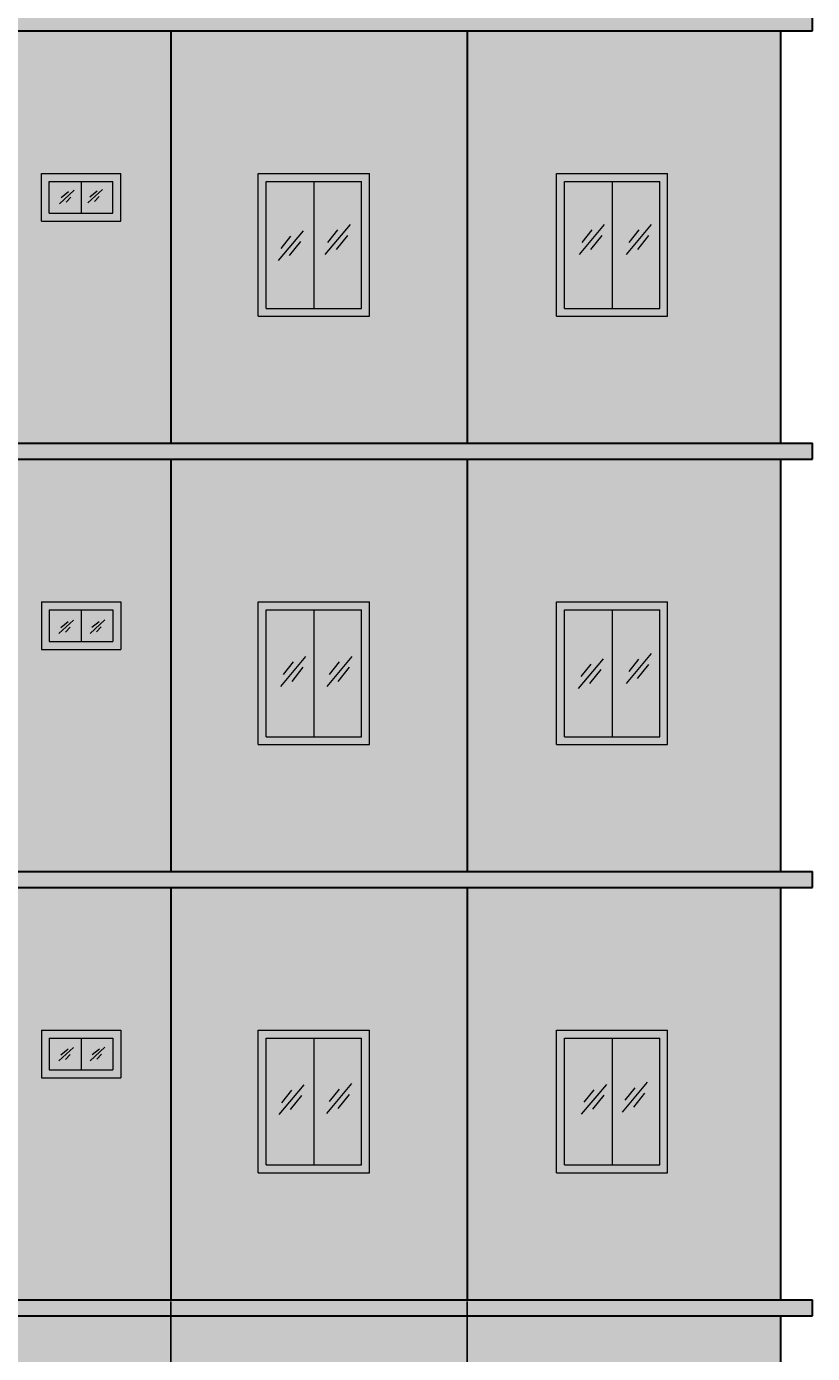
# Model space of a CAD drawing. Units: inches. Extents: x 2391 to 16591, y 7259 to 10239.
# Tile 6 of 27: x 2644 to 2941, y 7745 to 8247. Entities that reach past the tile are written whole.
import ezdxf

# ---------------------------------------------------------------- set-up
doc = ezdxf.new("R2010")
doc.units = ezdxf.units.IN
for name, color, linetype, lineweight in [('A-ANNO-DIMS', 4, 'Continuous', 18), ('A-ELEV', 7, 'Continuous', 30), ('A-ELEV-GLAZ', 4, 'Continuous', 18), ('A-ELEV-GLAZ-PATT', 141, 'Continuous', 13), ('A-ELEV-PATT', 8, 'Continuous', 13), ('A-ELEV-SURF-PATT', 253, 'Continuous', 13)]:
    doc.layers.add(name, color=color, linetype=linetype, lineweight=lineweight)
doc.styles.get("Standard").update_dxf_attribs({"font": 'arial.ttf'})
doc.dimstyles.new('ISO-25', dxfattribs={"dimtxt": 2.5, "dimasz": 2.5, "dimexe": 1.25, "dimexo": 0.625, "dimtad": 1, "dimdec": 0, "dimlunit": 3, "dimtxsty": 'Standard', "dimcen": 2.5, "dimadec": 0, "dimazin": 0, "dimtfac": 1, "dimtdec": 0, "dimtmove": 0, "dimatfit": 3, "dimfxl": 1, "dimarcsym": 0})

# ---------------------------------------------------------------- blocks, each defined once
blk = doc.blocks.new('GLASS-REFLECTION-VENT')
for p, q in [((0, 0), (5.55, 5.12)), ((0.7, 2.37), (3.45, 4.58)), ((2.48, 0.59), (4.26, 2.48))]:
    blk.add_line(p, q)
blk = doc.blocks.new('GLASS-REFLECTION-WINDOW')
for p, q in [((0, 0), (9.5, 11.3)), ((1, 4.52), (4.76, 9.26)), ((4.26, 1.91), (8.52, 7.21))]:
    blk.add_line(p, q)
blk = doc.blocks.new('*D79')
at = {"layer": 'A-ANNO-DIMS', "color": 0, "lineweight": -2, "transparency": 16777216}
for p, q in [((2707.14, 8351.94), (2436.96, 8351.94)), ((2438.21, 7591.44), (2438.21, 8349.44)), ((2490.64, 7588.94), (2436.96, 7588.94))]:
    blk.add_line(p, q, dxfattribs=at)
at = {"layer": 'A-ANNO-DIMS', "color": 0, "transparency": 16777216}
for points in [[(2437.8, 8349.44), (2438.63, 8349.44), (2438.21, 8351.94)], [(2437.8, 7591.44), (2438.63, 7591.44), (2438.21, 7588.94)]]:
    blk.add_solid(points, dxfattribs=at)
at = {"layer": 'Defpoints', "color": 0, "transparency": 16777216}
for p in [(2438.21, 8351.94), (2707.76, 8351.94), (2491.26, 7588.94)]:
    blk.add_point(p, dxfattribs=at)
at = {"layer": 'A-ANNO-DIMS', "color": 0, "transparency": 16777216, "insert": (2436.31, 7970.44), "char_height": 2.5, "attachment_point": 5, "rotation": 90}
blk.add_mtext('63\'-7"', dxfattribs=at)
blk = doc.blocks.new('*D80')
at = {"layer": 'A-ANNO-DIMS', "color": 0, "lineweight": -2, "transparency": 16777216}
for p, q in [((2698.76, 7764.31), (2698.76, 7540.64)), ((2497.26, 7758.31), (2497.26, 7540.64)), ((2499.76, 7541.89), (2696.26, 7541.89))]:
    blk.add_line(p, q, dxfattribs=at)
at = {"layer": 'A-ANNO-DIMS', "color": 0, "transparency": 16777216}
for points in [[(2499.76, 7542.3), (2499.76, 7541.47), (2497.26, 7541.89)], [(2696.26, 7542.3), (2696.26, 7541.47), (2698.76, 7541.89)]]:
    blk.add_solid(points, dxfattribs=at)
at = {"layer": 'Defpoints', "color": 0, "transparency": 16777216}
for p in [(2698.76, 7764.94), (2497.26, 7758.94), (2698.76, 7541.89)]:
    blk.add_point(p, dxfattribs=at)
at = {"layer": 'A-ANNO-DIMS', "color": 0, "transparency": 16777216, "insert": (2598.01, 7543.8), "char_height": 2.5, "attachment_point": 5}
blk.add_mtext('16\'-9 1/2"', dxfattribs=at)
blk = doc.blocks.new('*D81')
at = {"layer": 'A-ANNO-DIMS', "color": 0, "lineweight": -2, "transparency": 16777216}
for p, q in [((2698.76, 7764.31), (2698.76, 7540.64)), ((2810.76, 7764.31), (2810.76, 7540.64)), ((2701.26, 7541.89), (2808.26, 7541.89))]:
    blk.add_line(p, q, dxfattribs=at)
at = {"layer": 'A-ANNO-DIMS', "color": 0, "transparency": 16777216}
for points in [[(2701.26, 7542.3), (2701.26, 7541.47), (2698.76, 7541.89)], [(2808.26, 7542.3), (2808.26, 7541.47), (2810.76, 7541.89)]]:
    blk.add_solid(points, dxfattribs=at)
at = {"layer": 'Defpoints', "color": 0, "transparency": 16777216}
for p in [(2698.76, 7764.94), (2810.76, 7764.94), (2810.76, 7541.89)]:
    blk.add_point(p, dxfattribs=at)
at = {"layer": 'A-ANNO-DIMS', "color": 0, "transparency": 16777216, "insert": (2754.76, 7543.79), "char_height": 2.5, "attachment_point": 5}
blk.add_mtext('9\'-4"', dxfattribs=at)

msp = doc.modelspace()

# ---------------------------------------------------------------- hatches: boundary and pattern name
at = {"layer": 'A-ELEV-GLAZ-PATT'}
h = msp.add_hatch(color=256, dxfattribs=at)
h.dxf.hatch_style = 1
h.paths.add_polyline_path([(2679.76, 8190.94), (2649.76, 8190.94), (2649.76, 8172.94), (2679.76, 8172.94)])
h.paths.add_polyline_path([(2676.76, 8187.94), (2676.76, 8175.94), (2652.76, 8175.94), (2652.76, 8187.94)], flags=16)
h.paths.add_polyline_path([(2731.76, 8190.94), (2731.76, 8136.94), (2773.76, 8136.94), (2773.76, 8190.94)])
h.paths.add_polyline_path([(2770.76, 8187.94), (2770.76, 8139.94), (2734.76, 8139.94), (2734.76, 8187.94)], flags=16)
h.paths.add_polyline_path([(2886.51, 8190.94), (2844.51, 8190.94), (2844.51, 8136.94), (2886.51, 8136.94)])
h.paths.add_polyline_path([(2883.51, 8187.94), (2883.51, 8139.94), (2847.51, 8139.94), (2847.51, 8187.94)], flags=16)
h.paths.add_polyline_path([(2649.76, 8028.94), (2649.76, 8010.94), (2679.76, 8010.94), (2679.76, 8028.94)])
h.paths.add_polyline_path([(2676.76, 8025.94), (2676.76, 8013.94), (2652.76, 8013.94), (2652.76, 8025.94)], flags=16)
h.paths.add_polyline_path([(2731.76, 8028.94), (2731.76, 7974.94), (2773.76, 7974.94), (2773.76, 8028.94)])
h.paths.add_polyline_path([(2770.76, 8025.94), (2770.76, 7977.94), (2734.76, 7977.94), (2734.76, 8025.94)], flags=16)
h.paths.add_polyline_path([(2844.51, 8028.94), (2844.51, 7974.94), (2886.51, 7974.94), (2886.51, 8028.94)])
h.paths.add_polyline_path([(2847.51, 8025.94), (2883.51, 8025.94), (2883.51, 7977.94), (2847.51, 7977.94)], flags=16)
h.paths.add_polyline_path([(2679.76, 7866.94), (2649.76, 7866.94), (2649.76, 7848.94), (2679.76, 7848.94)])
h.paths.add_polyline_path([(2676.76, 7863.94), (2676.76, 7851.94), (2652.76, 7851.94), (2652.76, 7863.94)], flags=16)
h.paths.add_polyline_path([(2773.76, 7866.94), (2731.76, 7866.94), (2731.76, 7812.94), (2773.76, 7812.94)])
h.paths.add_polyline_path([(2734.76, 7863.94), (2770.76, 7863.94), (2770.76, 7815.94), (2734.76, 7815.94)], flags=16)
h.paths.add_polyline_path([(2844.51, 7866.94), (2844.51, 7812.94), (2886.51, 7812.94), (2886.51, 7866.94)])
h.paths.add_polyline_path([(2847.51, 7863.94), (2883.51, 7863.94), (2883.51, 7815.94), (2847.51, 7815.94)], flags=16)
h = msp.add_hatch(color=256, dxfattribs=at)
h.dxf.hatch_style = 1
h.paths.add_polyline_path([(2664.76, 8187.94), (2652.76, 8187.94), (2652.76, 8175.94), (2664.76, 8175.94)])
h.paths.add_polyline_path([(2676.76, 8187.94), (2664.76, 8187.94), (2664.76, 8175.94), (2676.76, 8175.94)])
h.paths.add_polyline_path([(2752.76, 8187.94), (2734.76, 8187.94), (2734.76, 8139.94), (2752.76, 8139.94)])
h.paths.add_polyline_path([(2770.76, 8187.94), (2752.76, 8187.94), (2752.76, 8139.94), (2770.76, 8139.94)])
h.paths.add_polyline_path([(2865.51, 8187.94), (2847.51, 8187.94), (2847.51, 8139.94), (2865.51, 8139.94)])
h.paths.add_polyline_path([(2883.51, 8187.94), (2865.51, 8187.94), (2865.51, 8139.94), (2883.51, 8139.94)])
h.paths.add_polyline_path([(2664.76, 8025.94), (2652.76, 8025.94), (2652.76, 8013.94), (2664.76, 8013.94)])
h.paths.add_polyline_path([(2676.76, 8025.94), (2664.76, 8025.94), (2664.76, 8013.94), (2676.76, 8013.94)])
h.paths.add_polyline_path([(2752.76, 8025.94), (2734.76, 8025.94), (2734.76, 7977.94), (2752.76, 7977.94)])
h.paths.add_polyline_path([(2770.76, 8025.94), (2752.76, 8025.94), (2752.76, 7977.94), (2770.76, 7977.94)])
h.paths.add_polyline_path([(2865.51, 8025.94), (2847.51, 8025.94), (2847.51, 7977.94), (2865.51, 7977.94)])
h.paths.add_polyline_path([(2883.51, 8025.94), (2865.51, 8025.94), (2865.51, 7977.94), (2883.51, 7977.94)])
h.paths.add_polyline_path([(2664.76, 7863.94), (2652.76, 7863.94), (2652.76, 7851.94), (2664.76, 7851.94)])
h.paths.add_polyline_path([(2676.76, 7863.94), (2664.76, 7863.94), (2664.76, 7851.94), (2676.76, 7851.94)])
h.paths.add_polyline_path([(2752.76, 7863.94), (2734.76, 7863.94), (2734.76, 7815.94), (2752.76, 7815.94)])
h.paths.add_polyline_path([(2770.76, 7863.94), (2752.76, 7863.94), (2752.76, 7815.94), (2770.76, 7815.94)])
h.paths.add_polyline_path([(2865.51, 7863.94), (2847.51, 7863.94), (2847.51, 7815.94), (2865.51, 7815.94)])
h.paths.add_polyline_path([(2883.51, 7863.94), (2865.51, 7863.94), (2865.51, 7815.94), (2883.51, 7815.94)])
at = {"layer": 'A-ELEV-PATT'}
h = msp.add_hatch(dxfattribs=at)
h.set_pattern_fill('TRIANG', color=256)
h.paths.add_polyline_path([(2698.76, 8244.94), (2497.26, 8244.94), (2497.26, 8088.94), (2698.76, 8088.94)])
h.paths.add_polyline_path([(2649.76, 8172.94), (2649.76, 8190.94), (2679.76, 8190.94), (2679.76, 8172.94)], flags=16)
h.paths.add_polyline_path([(2652.76, 8175.94), (2652.76, 8187.94), (2676.76, 8187.94), (2676.76, 8175.94)], flags=0)
h.paths.add_polyline_path([(2497.26, 8082.94), (2497.26, 7926.94), (2698.76, 7926.94), (2698.76, 8082.94)])
h.paths.add_polyline_path([(2649.76, 8028.94), (2679.76, 8028.94), (2679.76, 8010.94), (2649.76, 8010.94)], flags=16)
h.paths.add_polyline_path([(2652.76, 8025.94), (2676.76, 8025.94), (2676.76, 8013.94), (2652.76, 8013.94)], flags=0)
h.paths.add_polyline_path([(2497.26, 7920.94), (2497.26, 7764.94), (2698.76, 7764.94), (2698.76, 7920.94)])
h.paths.add_polyline_path([(2649.76, 7866.94), (2679.76, 7866.94), (2679.76, 7848.94), (2649.76, 7848.94)], flags=16)
h.paths.add_polyline_path([(2652.76, 7863.94), (2676.76, 7863.94), (2676.76, 7851.94), (2652.76, 7851.94)], flags=0)
h = msp.add_hatch(dxfattribs=at)
h.set_pattern_fill('STARS', color=256)
h.paths.add_polyline_path([(2810.76, 7920.94), (2698.76, 7920.94), (2698.76, 7764.94), (2810.76, 7764.94)])
h.paths.add_polyline_path([(2773.76, 7812.94), (2731.76, 7812.94), (2731.76, 7866.94), (2773.76, 7866.94)], flags=16)
h.paths.add_polyline_path([(2770.76, 7815.94), (2734.76, 7815.94), (2734.76, 7863.94), (2770.76, 7863.94)], flags=0)
h.paths.add_polyline_path([(2810.76, 8082.94), (2698.76, 8082.94), (2698.76, 7926.94), (2810.76, 7926.94)])
h.paths.add_polyline_path([(2773.76, 7974.94), (2731.76, 7974.94), (2731.76, 8028.94), (2773.76, 8028.94)], flags=16)
h.paths.add_polyline_path([(2770.76, 7977.94), (2734.76, 7977.94), (2734.76, 8025.94), (2770.76, 8025.94)], flags=0)
h.paths.add_polyline_path([(2810.76, 8244.94), (2698.76, 8244.94), (2698.76, 8088.94), (2810.76, 8088.94)])
h.paths.add_polyline_path([(2773.76, 8136.94), (2731.76, 8136.94), (2731.76, 8190.94), (2773.76, 8190.94)], flags=16)
h.paths.add_polyline_path([(2770.76, 8139.94), (2734.76, 8139.94), (2734.76, 8187.94), (2770.76, 8187.94)], flags=0)
h = msp.add_hatch(dxfattribs=at)
h.set_pattern_fill('STARS', color=256)
h.paths.add_polyline_path([(2929.26, 8244.94), (2810.76, 8244.94), (2810.76, 8088.94), (2929.26, 8088.94)])
h.paths.add_polyline_path([(2886.51, 8136.94), (2844.51, 8136.94), (2844.51, 8190.94), (2886.51, 8190.94)], flags=16)
h.paths.add_polyline_path([(2883.51, 8139.94), (2847.51, 8139.94), (2847.51, 8187.94), (2883.51, 8187.94)], flags=0)
h.paths.add_polyline_path([(2929.26, 8082.94), (2810.76, 8082.94), (2810.76, 7926.94), (2929.26, 7926.94)])
h.paths.add_polyline_path([(2886.51, 7974.94), (2844.51, 7974.94), (2844.51, 8028.94), (2886.51, 8028.94)], flags=16)
h.paths.add_polyline_path([(2883.51, 7977.94), (2847.51, 7977.94), (2847.51, 8025.94), (2883.51, 8025.94)], flags=0)
h.paths.add_polyline_path([(2929.26, 7920.94), (2810.76, 7920.94), (2810.76, 7764.94), (2929.26, 7764.94)])
h.paths.add_polyline_path([(2886.51, 7812.94), (2844.51, 7812.94), (2844.51, 7866.94), (2886.51, 7866.94)], flags=16)
h.paths.add_polyline_path([(2883.51, 7815.94), (2847.51, 7815.94), (2847.51, 7863.94), (2883.51, 7863.94)], flags=0)
at = {"layer": 'A-ELEV-SURF-PATT'}
h = msp.add_hatch(color=256, dxfattribs=at)
h.dxf.hatch_style = 1
h.paths.add_polyline_path([(2941.26, 7764.94), (2485.26, 7764.94), (2485.26, 7758.94), (2941.26, 7758.94)])
h.paths.add_polyline_path([(2941.26, 7920.94), (2941.26, 7926.94), (2485.26, 7926.94), (2485.26, 7920.94)])
h.paths.add_polyline_path([(2941.26, 8082.94), (2941.26, 8088.94), (2485.26, 8088.94), (2485.26, 8082.94)])
h.paths.add_polyline_path([(2485.26, 8250.94), (2485.26, 8244.94), (2941.26, 8244.94), (2941.26, 8250.94)])
h.paths.add_polyline_path([(2707.76, 8351.94), (2707.76, 8346.94), (2908.26, 8346.94), (2908.26, 8351.94)])
h = msp.add_hatch(color=256, dxfattribs=at)
h.dxf.hatch_style = 1
h.paths.add_polyline_path([(2929.26, 7758.94), (2497.26, 7758.94), (2497.26, 7715.94), (2690.26, 7715.94), (2690.26, 7724.94), (2685.26, 7724.94), (2685.26, 7729.94), (2704.26, 7729.94), (2704.26, 7724.94), (2699.26, 7724.94), (2699.26, 7695.78), (2701.76, 7695.78), (2701.76, 7697.78), (2704.26, 7697.78), (2704.26, 7722.94), (2773.26, 7722.94), (2773.26, 7607.94), (2704.26, 7607.94), (2704.26, 7602.94), (2843.26, 7602.94), (2843.26, 7607.94), (2774.26, 7607.94), (2774.26, 7722.94), (2843.26, 7722.94), (2843.26, 7697.78), (2845.76, 7697.78), (2845.76, 7695.78), (2848.26, 7695.78), (2848.26, 7724.94), (2843.26, 7724.94), (2843.26, 7729.94), (2862.26, 7729.94), (2862.26, 7724.94), (2857.26, 7724.94), (2857.26, 7715.94), (2929.26, 7715.94)])
h.paths.add_polyline_path([(2848.26, 7693.78), (2845.76, 7693.78), (2845.76, 7691.78), (2843.26, 7691.78), (2843.26, 7637.65), (2845.76, 7637.65), (2845.76, 7635.65), (2848.26, 7635.65)], flags=17)
h.paths.add_polyline_path([(2848.26, 7633.65), (2845.76, 7633.65), (2845.76, 7631.65), (2843.26, 7631.65), (2843.26, 7602.94), (2848.26, 7602.94)], flags=17)
h.paths.add_polyline_path([(2704.26, 7631.65), (2701.76, 7631.65), (2701.76, 7633.65), (2699.26, 7633.65), (2699.26, 7602.94), (2704.26, 7602.94), (2704.26, 7607.94)], flags=17)
h.paths.add_polyline_path([(2704.26, 7691.78), (2701.76, 7691.78), (2701.76, 7693.78), (2699.26, 7693.78), (2699.26, 7635.65), (2701.76, 7635.65), (2701.76, 7637.65), (2704.26, 7637.65)], flags=17)

# ---------------------------------------------------------------- linework, layer by layer
at = {"layer": 'A-ELEV'}
for p, q in [((2941.26, 8244.94), (2941.26, 8250.94)), ((2485.26, 8244.94), (2941.26, 8244.94)), ((2698.76, 8244.94), (2698.76, 8088.94)), ((2810.76, 8244.94), (2810.76, 8088.94)), ((2929.26, 8088.94), (2929.26, 8244.94)), ((2485.26, 8088.94), (2941.26, 8088.94)), ((2941.26, 8082.94), (2941.26, 8088.94)), ((2485.26, 8082.94), (2941.26, 8082.94)), ((2698.76, 8082.94), (2698.76, 7926.94)), ((2810.76, 8082.94), (2810.76, 7926.94)), ((2929.26, 7926.94), (2929.26, 8082.94)), ((2485.26, 7926.94), (2941.26, 7926.94)), ((2941.26, 7920.94), (2941.26, 7926.94)), ((2485.26, 7920.94), (2941.26, 7920.94)), ((2698.76, 7920.94), (2698.76, 7764.94)), ((2810.76, 7920.94), (2810.76, 7764.94)), ((2929.26, 7764.94), (2929.26, 7920.94)), ((2485.26, 7764.94), (2941.26, 7764.94)), ((2941.26, 7758.94), (2941.26, 7764.94)), ((2485.26, 7758.94), (2941.26, 7758.94)), ((2929.26, 7593.94), (2929.26, 7758.94))]:
    msp.add_line(p, q, dxfattribs=at)
at = {"layer": 'A-ELEV-GLAZ'}
for p, q in [((2649.76, 8190.94), (2679.76, 8190.94)), ((2649.76, 8172.94), (2649.76, 8190.94)), ((2679.76, 8172.94), (2679.76, 8190.94)), ((2731.76, 8190.94), (2773.76, 8190.94)), ((2731.76, 8136.94), (2731.76, 8190.94)), ((2773.76, 8136.94), (2773.76, 8190.94)), ((2844.51, 8190.94), (2886.51, 8190.94)), ((2844.51, 8136.94), (2844.51, 8190.94)), ((2886.51, 8136.94), (2886.51, 8190.94)), ((2652.76, 8187.94), (2676.76, 8187.94)), ((2652.76, 8175.94), (2652.76, 8187.94)), ((2664.76, 8187.94), (2664.76, 8175.94)), ((2676.76, 8175.94), (2676.76, 8187.94)), ((2734.76, 8187.94), (2770.76, 8187.94)), ((2734.76, 8139.94), (2734.76, 8187.94)), ((2752.76, 8187.94), (2752.76, 8139.94)), ((2770.76, 8139.94), (2770.76, 8187.94)), ((2847.51, 8187.94), (2883.51, 8187.94)), ((2847.51, 8139.94), (2847.51, 8187.94)), ((2865.51, 8187.94), (2865.51, 8139.94)), ((2883.51, 8139.94), (2883.51, 8187.94)), ((2652.76, 8175.94), (2676.76, 8175.94)), ((2649.76, 8172.94), (2679.76, 8172.94)), ((2731.76, 8136.94), (2773.76, 8136.94)), ((2734.76, 8139.94), (2770.76, 8139.94)), ((2844.51, 8136.94), (2886.51, 8136.94)), ((2847.51, 8139.94), (2883.51, 8139.94)), ((2649.76, 8028.94), (2679.76, 8028.94)), ((2649.76, 8028.94), (2649.76, 8010.94)), ((2652.76, 8025.94), (2676.76, 8025.94)), ((2652.76, 8025.94), (2652.76, 8013.94)), ((2664.76, 8025.94), (2664.76, 8013.94)), ((2676.76, 8025.94), (2676.76, 8013.94)), ((2679.76, 8028.94), (2679.76, 8010.94)), ((2731.76, 8028.94), (2773.76, 8028.94)), ((2731.76, 7974.94), (2731.76, 8028.94)), ((2734.76, 8025.94), (2770.76, 8025.94)), ((2734.76, 7977.94), (2734.76, 8025.94)), ((2752.76, 8025.94), (2752.76, 7977.94)), ((2770.76, 7977.94), (2770.76, 8025.94)), ((2773.76, 7974.94), (2773.76, 8028.94)), ((2844.51, 8028.94), (2886.51, 8028.94)), ((2844.51, 7974.94), (2844.51, 8028.94)), ((2847.51, 8025.94), (2883.51, 8025.94)), ((2847.51, 7977.94), (2847.51, 8025.94)), ((2865.51, 8025.94), (2865.51, 7977.94)), ((2883.51, 7977.94), (2883.51, 8025.94)), ((2886.51, 7974.94), (2886.51, 8028.94)), ((2649.76, 8010.94), (2679.76, 8010.94)), ((2652.76, 8013.94), (2676.76, 8013.94)), ((2731.76, 7974.94), (2773.76, 7974.94)), ((2734.76, 7977.94), (2770.76, 7977.94)), ((2844.51, 7974.94), (2886.51, 7974.94)), ((2847.51, 7977.94), (2883.51, 7977.94)), ((2649.76, 7866.94), (2679.76, 7866.94)), ((2649.76, 7866.94), (2649.76, 7848.94)), ((2679.76, 7866.94), (2679.76, 7848.94)), ((2731.76, 7812.94), (2731.76, 7866.94)), ((2731.76, 7866.94), (2773.76, 7866.94)), ((2773.76, 7812.94), (2773.76, 7866.94)), ((2844.51, 7812.94), (2844.51, 7866.94)), ((2844.51, 7866.94), (2886.51, 7866.94)), ((2886.51, 7812.94), (2886.51, 7866.94)), ((2652.76, 7863.94), (2676.76, 7863.94)), ((2652.76, 7863.94), (2652.76, 7851.94)), ((2664.76, 7863.94), (2664.76, 7851.94)), ((2676.76, 7863.94), (2676.76, 7851.94)), ((2734.76, 7815.94), (2734.76, 7863.94)), ((2734.76, 7863.94), (2770.76, 7863.94)), ((2752.76, 7863.94), (2752.76, 7815.94)), ((2770.76, 7815.94), (2770.76, 7863.94)), ((2847.51, 7815.94), (2847.51, 7863.94)), ((2847.51, 7863.94), (2883.51, 7863.94)), ((2865.51, 7863.94), (2865.51, 7815.94)), ((2883.51, 7815.94), (2883.51, 7863.94)), ((2652.76, 7851.94), (2676.76, 7851.94)), ((2649.76, 7848.94), (2679.76, 7848.94)), ((2734.76, 7815.94), (2770.76, 7815.94)), ((2847.51, 7815.94), (2883.51, 7815.94)), ((2731.76, 7812.94), (2773.76, 7812.94)), ((2844.51, 7812.94), (2886.51, 7812.94))]:
    msp.add_line(p, q, dxfattribs=at)

# ---------------------------------------------------------------- block references
for name, p in [('GLASS-REFLECTION-VENT', (2656.59, 8179.52)), ('GLASS-REFLECTION-VENT', (2667.34, 8179.79)), ('GLASS-REFLECTION-WINDOW', (2757.09, 8160.35)), ('GLASS-REFLECTION-WINDOW', (2853.2, 8160.35)), ('GLASS-REFLECTION-WINDOW', (2870.93, 8160.35)), ('GLASS-REFLECTION-WINDOW', (2739.36, 8158.01)), ('GLASS-REFLECTION-VENT', (2656.38, 8016.91)), ('GLASS-REFLECTION-VENT', (2668.15, 8016.97)), ('GLASS-REFLECTION-WINDOW', (2740.27, 7996.96)), ('GLASS-REFLECTION-WINDOW', (2757.74, 7996.96)), ('GLASS-REFLECTION-WINDOW', (2852.81, 7996.12)), ('GLASS-REFLECTION-WINDOW', (2870.92, 7998.04)), ('GLASS-REFLECTION-VENT', (2656.38, 7855.29)), ('GLASS-REFLECTION-VENT', (2668.23, 7855.35)), ('GLASS-REFLECTION-WINDOW', (2739.65, 7834.98)), ('GLASS-REFLECTION-WINDOW', (2757.68, 7835.4)), ('GLASS-REFLECTION-WINDOW', (2854.01, 7835.13)), ('GLASS-REFLECTION-WINDOW', (2869.43, 7835.92))]:
    msp.add_blockref(name, p, dxfattribs=at)

# ---------------------------------------------------------------- dimensions: what is measured, and where the dimension line sits
at = {"layer": 'A-ANNO-DIMS'}
dim = msp.add_linear_dim(base=(2438.21, 8351.94), p1=(2491.26, 7588.94), p2=(2707.76, 8351.94), angle=90, dimstyle='ISO-25', override={"dimdec": 1, "dimlfac": 1, "dimrnd": 0, "dimzin": 1, "dimdsep": 46, "dimlunit": 4, "dimfrac": 2}, dxfattribs=at)
dim.commit()
dim.dimension.update_dxf_attribs({"geometry": '*D79', "text_midpoint": (2436.31, 7970.44)})
for base, p1, p2, picture, middle in [((2698.76, 7541.89), (2497.26, 7758.94), (2698.76, 7764.94), '*D80', (2598.01, 7543.8)), ((2810.76, 7541.89), (2698.76, 7764.94), (2810.76, 7764.94), '*D81', (2754.76, 7543.79))]:
    dim = msp.add_linear_dim(base=base, p1=p1, p2=p2, dimstyle='ISO-25', override={"dimdec": 1, "dimlfac": 1, "dimrnd": 0, "dimzin": 1, "dimdsep": 46, "dimlunit": 4, "dimfrac": 2}, dxfattribs=at)
    dim.commit()
    dim.dimension.update_dxf_attribs({"geometry": picture, "text_midpoint": middle})

doc.saveas('drawing.dxf')
